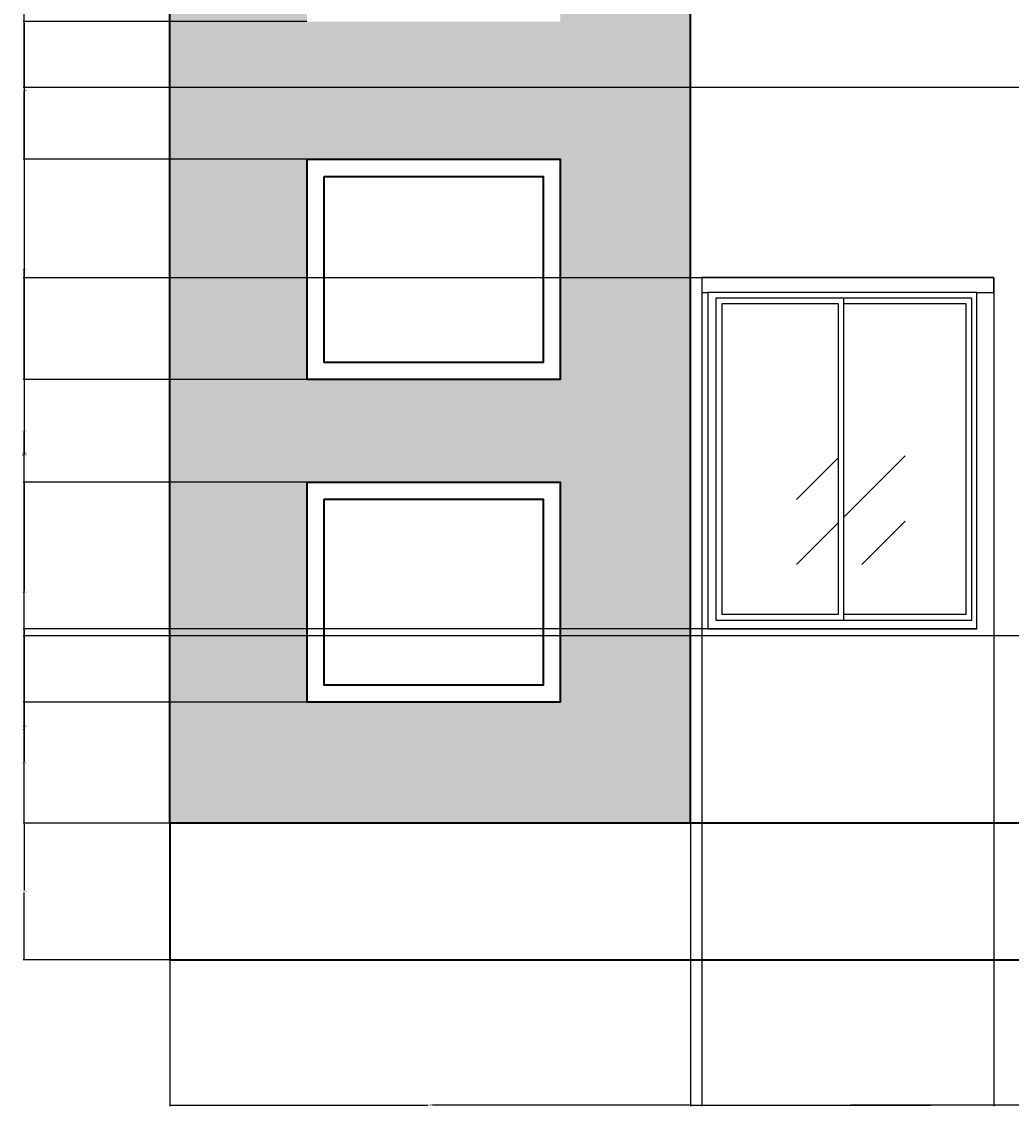
# Model space of a CAD drawing. Units: inches. Extents: x 93 to 565, y 123 to 656.
# Tile 1 of 18: x 93 to 267, y 134 to 324. Entities that reach past the tile are written whole.
import ezdxf

# ---------------------------------------------------------------- set-up
doc = ezdxf.new("R2010")
doc.units = ezdxf.units.IN
doc.header["$MEASUREMENT"] = 0
for name, color, linetype, lineweight in [('A-ANNO-DIMS', 2, 'Continuous', 18), ('A-ELEV', 7, 'Continuous', 35), ('A-GLAZ', 4, 'Continuous', 25), ('A-WALL-PATT', 8, 'Continuous', 13)]:
    doc.layers.add(name, color=color, linetype=linetype, lineweight=lineweight)
doc.styles.get("Standard").update_dxf_attribs({"font": 'arial.ttf'})
doc.dimstyles.get("Standard").update_dxf_attribs({"dimtxt": 0.18, "dimasz": 0.18, "dimexe": 0.18, "dimexo": 0.0625, "dimgap": 0.09, "dimtad": 0, "dimtih": 1, "dimtoh": 1, "dimdec": 4, "dimzin": 0, "dimdsep": 46, "dimtxsty": 'Standard', "dimcen": 0.09, "dimadec": 0, "dimazin": 0, "dimtfac": 1, "dimtdec": 4, "dimtofl": 0, "dimtmove": 0, "dimatfit": 3, "dimfxl": 1, "dimtolj": 1, "dimtzin": 0, "dimarcsym": 0})

# ---------------------------------------------------------------- blocks, each defined once
blk = doc.blocks.new('*U6')
for p, q in [((38.1, 38.1), (38.1, 1476.3)), ((38.1, 1476.3), (607.2, 1476.3)), ((607.2, 38.1), (607.2, 1476.3)), ((607.2, 1476.3), (1176.3, 1476.3)), ((1176.3, 1476.3), (1176.3, 38.1)), ((607.2, 38.1), (38.1, 38.1)), ((1176.3, 38.1), (607.2, 38.1))]:
    blk.add_line(p, q)
blk.add_lwpolyline([(0, 0), (1200, 0), (1200, 1500), (0, 1500)], close=True)
for points in [[(581.8, 1450.9), (581.8, 63.5), (63.5, 63.5), (63.5, 1450.9), (581.8, 1450.9)], [(607.2, 1450.9), (1150.9, 1450.9), (1150.9, 63.5), (607.2, 63.5)]]:
    blk.add_lwpolyline(points)
blk = doc.blocks.new('*D27')
at = {"layer": 'A-ANNO-DIMS', "color": 0, "lineweight": -2, "transparency": 16777216}
for p, q in [((210.54, 519.04), (210.54, 134)), ((119.08, 159.67), (119.08, 134)), ((119.26, 134.18), (164.42, 134.18)), ((210.36, 134.18), (165.21, 134.18))]:
    blk.add_line(p, q, dxfattribs=at)
at = {"layer": 'A-ANNO-DIMS', "color": 0, "transparency": 16777216}
for points in [[(119.26, 134.21), (119.26, 134.15), (119.08, 134.18)], [(210.36, 134.21), (210.36, 134.15), (210.54, 134.18)]]:
    blk.add_solid(points, dxfattribs=at)
at = {"layer": 'Defpoints', "color": 0, "transparency": 16777216}
for p in [(210.54, 519.1), (119.08, 159.73), (210.54, 134.18)]:
    blk.add_point(p, dxfattribs=at)
at = {"layer": 'A-ANNO-DIMS', "color": 0, "transparency": 16777216, "insert": (164.81, 134.18), "char_height": 0.18, "attachment_point": 5}
blk.add_mtext('\\A1;91.46', dxfattribs=at)
blk = doc.blocks.new('*D28')
at = {"layer": 'A-ANNO-DIMS', "color": 0, "lineweight": -2, "transparency": 16777216}
for p, q in [((210.54, 519.04), (210.54, 134)), ((295.69, 183.67), (295.69, 134)), ((210.72, 134.18), (252.72, 134.18)), ((295.51, 134.18), (253.51, 134.18))]:
    blk.add_line(p, q, dxfattribs=at)
at = {"layer": 'A-ANNO-DIMS', "color": 0, "transparency": 16777216}
for points in [[(210.72, 134.21), (210.72, 134.15), (210.54, 134.18)], [(295.51, 134.21), (295.51, 134.15), (295.69, 134.18)]]:
    blk.add_solid(points, dxfattribs=at)
at = {"layer": 'Defpoints', "color": 0, "transparency": 16777216}
for p in [(210.54, 519.1), (295.69, 183.73), (295.69, 134.18)]:
    blk.add_point(p, dxfattribs=at)
at = {"layer": 'A-ANNO-DIMS', "color": 0, "transparency": 16777216, "insert": (253.12, 134.18), "char_height": 0.18, "attachment_point": 5}
blk.add_mtext('\\A1;85.14', dxfattribs=at)
blk = doc.blocks.new('*D31')
at = {"layer": 'A-ANNO-DIMS', "color": 0, "lineweight": -2, "transparency": 16777216}
for p, q in [((417.87, 630.4), (564.81, 630.4)), ((564.63, 630.22), (564.63, 395.25)), ((564.63, 159.91), (564.63, 394.89)), ((119.14, 159.73), (564.81, 159.73))]:
    blk.add_line(p, q, dxfattribs=at)
at = {"layer": 'A-ANNO-DIMS', "color": 0, "transparency": 16777216}
for points in [[(564.6, 630.22), (564.66, 630.22), (564.63, 630.4)], [(564.6, 159.91), (564.66, 159.91), (564.63, 159.73)]]:
    blk.add_solid(points, dxfattribs=at)
at = {"layer": 'Defpoints', "color": 0, "transparency": 16777216}
for p in [(417.81, 630.4), (564.63, 630.4), (119.08, 159.73)]:
    blk.add_point(p, dxfattribs=at)
at = {"layer": 'A-ANNO-DIMS', "color": 0, "transparency": 16777216, "insert": (564.63, 395.07), "char_height": 0.18, "attachment_point": 5}
blk.add_mtext('\\A1;470.7', dxfattribs=at)
blk = doc.blocks.new('*D32')
at = {"layer": 'A-ANNO-DIMS', "color": 0, "lineweight": -2, "transparency": 16777216}
for p, q in [((119.02, 183.73), (93.35, 183.73)), ((93.53, 183.55), (93.53, 171.91)), ((93.53, 159.91), (93.53, 171.55)), ((119.02, 159.73), (93.35, 159.73))]:
    blk.add_line(p, q, dxfattribs=at)
at = {"layer": 'A-ANNO-DIMS', "color": 0, "transparency": 16777216}
for points in [[(93.5, 183.55), (93.56, 183.55), (93.53, 183.73)], [(93.5, 159.91), (93.56, 159.91), (93.53, 159.73)]]:
    blk.add_solid(points, dxfattribs=at)
at = {"layer": 'Defpoints', "color": 0, "transparency": 16777216}
for p in [(93.53, 183.73), (119.08, 183.73), (119.08, 159.73)]:
    blk.add_point(p, dxfattribs=at)
at = {"layer": 'A-ANNO-DIMS', "color": 0, "transparency": 16777216, "insert": (93.53, 171.73), "char_height": 0.18, "attachment_point": 5}
blk.add_mtext('\\A1;24', dxfattribs=at)
blk = doc.blocks.new('*D33')
at = {"layer": 'A-ANNO-DIMS', "color": 0, "lineweight": -2, "transparency": 16777216}
for p, q in [((286.62, 312.95), (93.35, 312.95)), ((93.53, 312.77), (93.53, 248.52)), ((93.53, 183.91), (93.53, 248.16)), ((119.02, 183.73), (93.35, 183.73))]:
    blk.add_line(p, q, dxfattribs=at)
at = {"layer": 'A-ANNO-DIMS', "color": 0, "transparency": 16777216}
for points in [[(93.5, 312.77), (93.56, 312.77), (93.53, 312.95)], [(93.5, 183.91), (93.56, 183.91), (93.53, 183.73)]]:
    blk.add_solid(points, dxfattribs=at)
at = {"layer": 'Defpoints', "color": 0, "transparency": 16777216}
for p in [(93.53, 312.95), (286.69, 312.95), (119.08, 183.73)]:
    blk.add_point(p, dxfattribs=at)
at = {"layer": 'A-ANNO-DIMS', "color": 0, "transparency": 16777216, "insert": (93.53, 248.34), "char_height": 0.18, "attachment_point": 5}
blk.add_mtext('\\A1;129.22', dxfattribs=at)
blk = doc.blocks.new('*D34')
at = {"layer": 'A-ANNO-DIMS', "color": 0, "lineweight": -2, "transparency": 16777216}
for p, q in [((286.62, 363.73), (93.35, 363.73)), ((93.53, 363.55), (93.53, 338.52)), ((93.53, 313.13), (93.53, 338.16)), ((286.62, 312.95), (93.35, 312.95))]:
    blk.add_line(p, q, dxfattribs=at)
at = {"layer": 'A-ANNO-DIMS', "color": 0, "transparency": 16777216}
for points in [[(93.5, 363.55), (93.56, 363.55), (93.53, 363.73)], [(93.5, 313.13), (93.56, 313.13), (93.53, 312.95)]]:
    blk.add_solid(points, dxfattribs=at)
at = {"layer": 'Defpoints', "color": 0, "transparency": 16777216}
for p in [(93.53, 363.73), (286.69, 363.73), (286.69, 312.95)]:
    blk.add_point(p, dxfattribs=at)
at = {"layer": 'A-ANNO-DIMS', "color": 0, "transparency": 16777216, "insert": (93.53, 338.34), "char_height": 0.18, "attachment_point": 5}
blk.add_mtext('\\A1;50.78', dxfattribs=at)
blk = doc.blocks.new('*D38')
at = {"layer": 'A-ANNO-DIMS', "color": 0, "lineweight": -2, "transparency": 16777216}
for p, q in [((143.15, 204.96), (93.35, 204.96)), ((93.53, 204.78), (93.53, 194.53)), ((93.53, 183.91), (93.53, 194.16)), ((210.48, 183.73), (93.35, 183.73))]:
    blk.add_line(p, q, dxfattribs=at)
at = {"layer": 'A-ANNO-DIMS', "color": 0, "transparency": 16777216}
for points in [[(93.5, 204.78), (93.56, 204.78), (93.53, 204.96)], [(93.5, 183.91), (93.56, 183.91), (93.53, 183.73)]]:
    blk.add_solid(points, dxfattribs=at)
at = {"layer": 'Defpoints', "color": 0, "transparency": 16777216}
for p in [(93.53, 204.96), (143.21, 204.96), (210.54, 183.73)]:
    blk.add_point(p, dxfattribs=at)
at = {"layer": 'A-ANNO-DIMS', "color": 0, "transparency": 16777216, "insert": (93.53, 194.35), "char_height": 0.18, "attachment_point": 5}
blk.add_mtext('\\A1;21.226', dxfattribs=at)
blk = doc.blocks.new('*D39')
at = {"layer": 'A-ANNO-DIMS', "color": 0, "lineweight": -2, "transparency": 16777216}
for p, q in [((143.15, 243.64), (93.35, 243.64)), ((93.53, 243.46), (93.53, 224.48)), ((93.53, 205.14), (93.53, 224.12)), ((143.15, 204.96), (93.35, 204.96))]:
    blk.add_line(p, q, dxfattribs=at)
at = {"layer": 'A-ANNO-DIMS', "color": 0, "transparency": 16777216}
for points in [[(93.5, 243.46), (93.56, 243.46), (93.53, 243.64)], [(93.5, 205.14), (93.56, 205.14), (93.53, 204.96)]]:
    blk.add_solid(points, dxfattribs=at)
at = {"layer": 'Defpoints', "color": 0, "transparency": 16777216}
for p in [(93.53, 243.64), (143.21, 243.64), (143.21, 204.96)]:
    blk.add_point(p, dxfattribs=at)
at = {"layer": 'A-ANNO-DIMS', "color": 0, "transparency": 16777216, "insert": (93.53, 224.3), "char_height": 0.18, "attachment_point": 5}
blk.add_mtext('\\A1;38.685', dxfattribs=at)
blk = doc.blocks.new('*D40')
at = {"layer": 'A-ANNO-DIMS', "color": 0, "lineweight": -2, "transparency": 16777216}
for p, q in [((143.15, 261.64), (93.35, 261.64)), ((93.53, 261.46), (93.53, 252.82)), ((93.53, 243.82), (93.53, 252.46)), ((143.15, 243.64), (93.35, 243.64))]:
    blk.add_line(p, q, dxfattribs=at)
at = {"layer": 'A-ANNO-DIMS', "color": 0, "transparency": 16777216}
for points in [[(93.5, 261.46), (93.56, 261.46), (93.53, 261.64)], [(93.5, 243.82), (93.56, 243.82), (93.53, 243.64)]]:
    blk.add_solid(points, dxfattribs=at)
at = {"layer": 'Defpoints', "color": 0, "transparency": 16777216}
for p in [(93.53, 261.64), (143.21, 261.64), (143.21, 243.64)]:
    blk.add_point(p, dxfattribs=at)
at = {"layer": 'A-ANNO-DIMS', "color": 0, "transparency": 16777216, "insert": (93.53, 252.64), "char_height": 0.18, "attachment_point": 5}
blk.add_mtext('\\A1;17.995', dxfattribs=at)
blk = doc.blocks.new('*D41')
at = {"layer": 'A-ANNO-DIMS', "color": 0, "lineweight": -2, "transparency": 16777216}
for p, q in [((143.15, 300.32), (93.35, 300.32)), ((93.53, 300.14), (93.53, 281.16)), ((93.53, 261.82), (93.53, 280.8)), ((143.15, 261.64), (93.35, 261.64))]:
    blk.add_line(p, q, dxfattribs=at)
at = {"layer": 'A-ANNO-DIMS', "color": 0, "transparency": 16777216}
for points in [[(93.5, 300.14), (93.56, 300.14), (93.53, 300.32)], [(93.5, 261.82), (93.56, 261.82), (93.53, 261.64)]]:
    blk.add_solid(points, dxfattribs=at)
at = {"layer": 'Defpoints', "color": 0, "transparency": 16777216}
for p in [(93.53, 300.32), (143.21, 300.32), (143.21, 261.64)]:
    blk.add_point(p, dxfattribs=at)
at = {"layer": 'A-ANNO-DIMS', "color": 0, "transparency": 16777216, "insert": (93.53, 280.98), "char_height": 0.18, "attachment_point": 5}
blk.add_mtext('\\A1;38.685', dxfattribs=at)
blk = doc.blocks.new('*D42')
at = {"layer": 'A-ANNO-DIMS', "color": 0, "lineweight": -2, "transparency": 16777216}
for p, q in [((143.15, 324.49), (93.35, 324.49)), ((93.53, 324.31), (93.53, 312.59)), ((93.53, 300.5), (93.53, 312.22)), ((143.15, 300.32), (93.35, 300.32))]:
    blk.add_line(p, q, dxfattribs=at)
at = {"layer": 'A-ANNO-DIMS', "color": 0, "transparency": 16777216}
for points in [[(93.5, 324.31), (93.56, 324.31), (93.53, 324.49)], [(93.5, 300.5), (93.56, 300.5), (93.53, 300.32)]]:
    blk.add_solid(points, dxfattribs=at)
at = {"layer": 'Defpoints', "color": 0, "transparency": 16777216}
for p in [(93.53, 324.49), (143.21, 324.49), (143.21, 300.32)]:
    blk.add_point(p, dxfattribs=at)
at = {"layer": 'A-ANNO-DIMS', "color": 0, "transparency": 16777216, "insert": (93.53, 312.4), "char_height": 0.18, "attachment_point": 5}
blk.add_mtext('\\A1;24.16', dxfattribs=at)
blk = doc.blocks.new('*D43')
at = {"layer": 'A-ANNO-DIMS', "color": 0, "lineweight": -2, "transparency": 16777216}
for p, q in [((143.15, 363.17), (93.35, 363.17)), ((93.53, 362.99), (93.53, 344.01)), ((93.53, 324.67), (93.53, 343.65)), ((143.15, 324.49), (93.35, 324.49))]:
    blk.add_line(p, q, dxfattribs=at)
at = {"layer": 'A-ANNO-DIMS', "color": 0, "transparency": 16777216}
for points in [[(93.5, 362.99), (93.56, 362.99), (93.53, 363.17)], [(93.5, 324.67), (93.56, 324.67), (93.53, 324.49)]]:
    blk.add_solid(points, dxfattribs=at)
at = {"layer": 'Defpoints', "color": 0, "transparency": 16777216}
for p in [(93.53, 363.17), (143.21, 363.17), (143.21, 324.49)]:
    blk.add_point(p, dxfattribs=at)
at = {"layer": 'A-ANNO-DIMS', "color": 0, "transparency": 16777216, "insert": (93.53, 343.83), "char_height": 0.18, "attachment_point": 5}
blk.add_mtext('\\A1;38.685', dxfattribs=at)
blk = doc.blocks.new('*D52')
at = {"layer": 'A-ANNO-DIMS', "color": 0, "lineweight": -2, "transparency": 16777216}
for p, q in [((212.49, 279.47), (212.49, 134)), ((263.81, 279.47), (263.81, 134)), ((212.67, 134.18), (237.76, 134.18)), ((263.63, 134.18), (238.54, 134.18))]:
    blk.add_line(p, q, dxfattribs=at)
at = {"layer": 'A-ANNO-DIMS', "color": 0, "transparency": 16777216}
for points in [[(212.67, 134.21), (212.67, 134.15), (212.49, 134.18)], [(263.63, 134.21), (263.63, 134.15), (263.81, 134.18)]]:
    blk.add_solid(points, dxfattribs=at)
at = {"layer": 'Defpoints', "color": 0, "transparency": 16777216}
for p in [(212.49, 279.53), (263.81, 279.53), (263.81, 134.18)]:
    blk.add_point(p, dxfattribs=at)
at = {"layer": 'A-ANNO-DIMS', "color": 0, "transparency": 16777216, "insert": (238.15, 134.18), "char_height": 0.18, "attachment_point": 5}
blk.add_mtext('\\A1;51.33', dxfattribs=at)
blk = doc.blocks.new('*D53')
at = {"layer": 'A-ANNO-DIMS', "color": 0, "lineweight": -2, "transparency": 16777216}
for p, q in [((263.75, 279.53), (93.35, 279.53)), ((93.53, 279.35), (93.53, 248.87)), ((93.53, 218.03), (93.53, 248.51)), ((260.74, 217.85), (93.35, 217.85))]:
    blk.add_line(p, q, dxfattribs=at)
at = {"layer": 'A-ANNO-DIMS', "color": 0, "transparency": 16777216}
for points in [[(93.5, 279.35), (93.56, 279.35), (93.53, 279.53)], [(93.5, 218.03), (93.56, 218.03), (93.53, 217.85)]]:
    blk.add_solid(points, dxfattribs=at)
at = {"layer": 'Defpoints', "color": 0, "transparency": 16777216}
for p in [(93.53, 279.53), (263.81, 279.53), (260.8, 217.85)]:
    blk.add_point(p, dxfattribs=at)
at = {"layer": 'A-ANNO-DIMS', "color": 0, "transparency": 16777216, "insert": (93.53, 248.69), "char_height": 0.18, "attachment_point": 5}
blk.add_mtext('\\A1;61.68', dxfattribs=at)
blk = doc.blocks.new('*D54')
at = {"layer": 'A-ANNO-DIMS', "color": 0, "lineweight": -2, "transparency": 16777216}
for p, q in [((213.49, 217.85), (93.35, 217.85)), ((93.53, 217.67), (93.53, 200.97)), ((93.53, 183.91), (93.53, 200.61)), ((210.48, 183.73), (93.35, 183.73))]:
    blk.add_line(p, q, dxfattribs=at)
at = {"layer": 'A-ANNO-DIMS', "color": 0, "transparency": 16777216}
for points in [[(93.5, 217.67), (93.56, 217.67), (93.53, 217.85)], [(93.5, 183.91), (93.56, 183.91), (93.53, 183.73)]]:
    blk.add_solid(points, dxfattribs=at)
at = {"layer": 'Defpoints', "color": 0, "transparency": 16777216}
for p in [(213.56, 217.85), (93.53, 183.73), (210.54, 183.73)]:
    blk.add_point(p, dxfattribs=at)
at = {"layer": 'A-ANNO-DIMS', "color": 0, "transparency": 16777216, "insert": (93.53, 200.79), "char_height": 0.18, "attachment_point": 5}
blk.add_mtext('\\A1;34.114', dxfattribs=at)
blk = doc.blocks.new('*D58')
at = {"layer": 'A-ANNO-DIMS', "color": 0, "lineweight": -2, "transparency": 16777216}
for p, q in [((309.68, 216.63), (93.35, 216.63)), ((93.53, 216.45), (93.53, 200.36)), ((93.53, 183.91), (93.53, 200)), ((295.62, 183.73), (93.35, 183.73))]:
    blk.add_line(p, q, dxfattribs=at)
at = {"layer": 'A-ANNO-DIMS', "color": 0, "transparency": 16777216}
for points in [[(93.5, 216.45), (93.56, 216.45), (93.53, 216.63)], [(93.5, 183.91), (93.56, 183.91), (93.53, 183.73)]]:
    blk.add_solid(points, dxfattribs=at)
at = {"layer": 'Defpoints', "color": 0, "transparency": 16777216}
for p in [(309.74, 216.63), (93.53, 183.73), (295.69, 183.73)]:
    blk.add_point(p, dxfattribs=at)
at = {"layer": 'A-ANNO-DIMS', "color": 0, "transparency": 16777216, "insert": (93.53, 200.18), "char_height": 0.18, "attachment_point": 5}
blk.add_mtext('\\A1;32.9', dxfattribs=at)
blk = doc.blocks.new('*D106')
at = {"layer": 'A-ANNO-DIMS', "color": 0, "lineweight": -2, "transparency": 16777216}
for p, q in [((210.54, 519.04), (210.54, 134)), ((119.08, 159.67), (119.08, 134)), ((119.26, 134.18), (164.35, 134.18)), ((210.36, 134.18), (165.28, 134.18))]:
    blk.add_line(p, q, dxfattribs=at)
at = {"layer": 'A-ANNO-DIMS', "color": 0, "transparency": 16777216}
for points in [[(119.26, 134.21), (119.26, 134.15), (119.08, 134.18)], [(210.36, 134.21), (210.36, 134.15), (210.54, 134.18)]]:
    blk.add_solid(points, dxfattribs=at)
at = {"layer": 'Defpoints', "color": 0, "transparency": 16777216}
for p in [(210.54, 519.1), (119.08, 159.73), (210.54, 134.18)]:
    blk.add_point(p, dxfattribs=at)
at = {"layer": 'A-ANNO-DIMS', "color": 0, "transparency": 16777216, "insert": (164.81, 134.18), "char_height": 0.18, "attachment_point": 5}
blk.add_mtext('\\A1;91.465', dxfattribs=at)
blk = doc.blocks.new('*D107')
at = {"layer": 'A-ANNO-DIMS', "color": 0, "lineweight": -2, "transparency": 16777216}
for p, q in [((210.54, 519.04), (210.54, 134)), ((295.69, 183.67), (295.69, 134)), ((210.72, 134.18), (252.65, 134.18)), ((295.51, 134.18), (253.58, 134.18))]:
    blk.add_line(p, q, dxfattribs=at)
at = {"layer": 'A-ANNO-DIMS', "color": 0, "transparency": 16777216}
for points in [[(210.72, 134.21), (210.72, 134.15), (210.54, 134.18)], [(295.51, 134.21), (295.51, 134.15), (295.69, 134.18)]]:
    blk.add_solid(points, dxfattribs=at)
at = {"layer": 'Defpoints', "color": 0, "transparency": 16777216}
for p in [(210.54, 519.1), (295.69, 183.73), (295.69, 134.18)]:
    blk.add_point(p, dxfattribs=at)
at = {"layer": 'A-ANNO-DIMS', "color": 0, "transparency": 16777216, "insert": (253.12, 134.18), "char_height": 0.18, "attachment_point": 5}
blk.add_mtext('\\A1;85.143', dxfattribs=at)
blk = doc.blocks.new('*D110')
at = {"layer": 'A-ANNO-DIMS', "color": 0, "lineweight": -2, "transparency": 16777216}
for p, q in [((417.87, 630.4), (564.81, 630.4)), ((564.63, 630.22), (564.63, 395.25)), ((564.63, 159.91), (564.63, 394.89)), ((119.14, 159.73), (564.81, 159.73))]:
    blk.add_line(p, q, dxfattribs=at)
at = {"layer": 'A-ANNO-DIMS', "color": 0, "transparency": 16777216}
for points in [[(564.6, 630.22), (564.66, 630.22), (564.63, 630.4)], [(564.6, 159.91), (564.66, 159.91), (564.63, 159.73)]]:
    blk.add_solid(points, dxfattribs=at)
at = {"layer": 'Defpoints', "color": 0, "transparency": 16777216}
for p in [(417.81, 630.4), (564.63, 630.4), (119.08, 159.73)]:
    blk.add_point(p, dxfattribs=at)
at = {"layer": 'A-ANNO-DIMS', "color": 0, "transparency": 16777216, "insert": (564.63, 395.07), "char_height": 0.18, "attachment_point": 5}
blk.add_mtext('\\A1;470.673', dxfattribs=at)
blk = doc.blocks.new('*D111')
at = {"layer": 'A-ANNO-DIMS', "color": 0, "lineweight": -2, "transparency": 16777216}
for p, q in [((119.02, 183.73), (93.35, 183.73)), ((93.53, 183.55), (93.53, 171.91)), ((93.53, 159.91), (93.53, 171.55)), ((119.02, 159.73), (93.35, 159.73))]:
    blk.add_line(p, q, dxfattribs=at)
at = {"layer": 'A-ANNO-DIMS', "color": 0, "transparency": 16777216}
for points in [[(93.5, 183.55), (93.56, 183.55), (93.53, 183.73)], [(93.5, 159.91), (93.56, 159.91), (93.53, 159.73)]]:
    blk.add_solid(points, dxfattribs=at)
at = {"layer": 'Defpoints', "color": 0, "transparency": 16777216}
for p in [(93.53, 183.73), (119.08, 183.73), (119.08, 159.73)]:
    blk.add_point(p, dxfattribs=at)
at = {"layer": 'A-ANNO-DIMS', "color": 0, "transparency": 16777216, "insert": (93.53, 171.73), "char_height": 0.18, "attachment_point": 5}
blk.add_mtext('\\A1;24.000', dxfattribs=at)
blk = doc.blocks.new('*D112')
at = {"layer": 'A-ANNO-DIMS', "color": 0, "lineweight": -2, "transparency": 16777216}
for p, q in [((286.62, 312.95), (93.35, 312.95)), ((93.53, 312.77), (93.53, 248.52)), ((93.53, 183.91), (93.53, 248.16)), ((119.02, 183.73), (93.35, 183.73))]:
    blk.add_line(p, q, dxfattribs=at)
at = {"layer": 'A-ANNO-DIMS', "color": 0, "transparency": 16777216}
for points in [[(93.5, 312.77), (93.56, 312.77), (93.53, 312.95)], [(93.5, 183.91), (93.56, 183.91), (93.53, 183.73)]]:
    blk.add_solid(points, dxfattribs=at)
at = {"layer": 'Defpoints', "color": 0, "transparency": 16777216}
for p in [(93.53, 312.95), (286.69, 312.95), (119.08, 183.73)]:
    blk.add_point(p, dxfattribs=at)
at = {"layer": 'A-ANNO-DIMS', "color": 0, "transparency": 16777216, "insert": (93.53, 248.34), "char_height": 0.18, "attachment_point": 5}
blk.add_mtext('\\A1;129.217', dxfattribs=at)
blk = doc.blocks.new('*D113')
at = {"layer": 'A-ANNO-DIMS', "color": 0, "lineweight": -2, "transparency": 16777216}
for p, q in [((286.62, 363.73), (93.35, 363.73)), ((93.53, 363.55), (93.53, 338.52)), ((93.53, 313.13), (93.53, 338.16)), ((286.62, 312.95), (93.35, 312.95))]:
    blk.add_line(p, q, dxfattribs=at)
at = {"layer": 'A-ANNO-DIMS', "color": 0, "transparency": 16777216}
for points in [[(93.5, 363.55), (93.56, 363.55), (93.53, 363.73)], [(93.5, 313.13), (93.56, 313.13), (93.53, 312.95)]]:
    blk.add_solid(points, dxfattribs=at)
at = {"layer": 'Defpoints', "color": 0, "transparency": 16777216}
for p in [(93.53, 363.73), (286.69, 363.73), (286.69, 312.95)]:
    blk.add_point(p, dxfattribs=at)
at = {"layer": 'A-ANNO-DIMS', "color": 0, "transparency": 16777216, "insert": (93.53, 338.34), "char_height": 0.18, "attachment_point": 5}
blk.add_mtext('\\A1;50.783', dxfattribs=at)
blk = doc.blocks.new('*D117')
at = {"layer": 'A-ANNO-DIMS', "color": 0, "lineweight": -2, "transparency": 16777216}
for p, q in [((143.15, 204.96), (93.35, 204.96)), ((93.53, 204.78), (93.53, 194.53)), ((93.53, 183.91), (93.53, 194.16)), ((210.48, 183.73), (93.35, 183.73))]:
    blk.add_line(p, q, dxfattribs=at)
at = {"layer": 'A-ANNO-DIMS', "color": 0, "transparency": 16777216}
for points in [[(93.5, 204.78), (93.56, 204.78), (93.53, 204.96)], [(93.5, 183.91), (93.56, 183.91), (93.53, 183.73)]]:
    blk.add_solid(points, dxfattribs=at)
at = {"layer": 'Defpoints', "color": 0, "transparency": 16777216}
for p in [(93.53, 204.96), (143.21, 204.96), (210.54, 183.73)]:
    blk.add_point(p, dxfattribs=at)
at = {"layer": 'A-ANNO-DIMS', "color": 0, "transparency": 16777216, "insert": (93.53, 194.35), "char_height": 0.18, "attachment_point": 5}
blk.add_mtext('\\A1;21.226', dxfattribs=at)
blk = doc.blocks.new('*D118')
at = {"layer": 'A-ANNO-DIMS', "color": 0, "lineweight": -2, "transparency": 16777216}
for p, q in [((143.15, 243.64), (93.35, 243.64)), ((93.53, 243.46), (93.53, 224.48)), ((93.53, 205.14), (93.53, 224.12)), ((143.15, 204.96), (93.35, 204.96))]:
    blk.add_line(p, q, dxfattribs=at)
at = {"layer": 'A-ANNO-DIMS', "color": 0, "transparency": 16777216}
for points in [[(93.5, 243.46), (93.56, 243.46), (93.53, 243.64)], [(93.5, 205.14), (93.56, 205.14), (93.53, 204.96)]]:
    blk.add_solid(points, dxfattribs=at)
at = {"layer": 'Defpoints', "color": 0, "transparency": 16777216}
for p in [(93.53, 243.64), (143.21, 243.64), (143.21, 204.96)]:
    blk.add_point(p, dxfattribs=at)
at = {"layer": 'A-ANNO-DIMS', "color": 0, "transparency": 16777216, "insert": (93.53, 224.3), "char_height": 0.18, "attachment_point": 5}
blk.add_mtext('\\A1;38.685', dxfattribs=at)
blk = doc.blocks.new('*D119')
at = {"layer": 'A-ANNO-DIMS', "color": 0, "lineweight": -2, "transparency": 16777216}
for p, q in [((143.15, 261.64), (93.35, 261.64)), ((93.53, 261.46), (93.53, 252.82)), ((93.53, 243.82), (93.53, 252.46)), ((143.15, 243.64), (93.35, 243.64))]:
    blk.add_line(p, q, dxfattribs=at)
at = {"layer": 'A-ANNO-DIMS', "color": 0, "transparency": 16777216}
for points in [[(93.5, 261.46), (93.56, 261.46), (93.53, 261.64)], [(93.5, 243.82), (93.56, 243.82), (93.53, 243.64)]]:
    blk.add_solid(points, dxfattribs=at)
at = {"layer": 'Defpoints', "color": 0, "transparency": 16777216}
for p in [(93.53, 261.64), (143.21, 261.64), (143.21, 243.64)]:
    blk.add_point(p, dxfattribs=at)
at = {"layer": 'A-ANNO-DIMS', "color": 0, "transparency": 16777216, "insert": (93.53, 252.64), "char_height": 0.18, "attachment_point": 5}
blk.add_mtext('\\A1;17.995', dxfattribs=at)
blk = doc.blocks.new('*D120')
at = {"layer": 'A-ANNO-DIMS', "color": 0, "lineweight": -2, "transparency": 16777216}
for p, q in [((143.15, 300.32), (93.35, 300.32)), ((93.53, 300.14), (93.53, 281.16)), ((93.53, 261.82), (93.53, 280.8)), ((143.15, 261.64), (93.35, 261.64))]:
    blk.add_line(p, q, dxfattribs=at)
at = {"layer": 'A-ANNO-DIMS', "color": 0, "transparency": 16777216}
for points in [[(93.5, 300.14), (93.56, 300.14), (93.53, 300.32)], [(93.5, 261.82), (93.56, 261.82), (93.53, 261.64)]]:
    blk.add_solid(points, dxfattribs=at)
at = {"layer": 'Defpoints', "color": 0, "transparency": 16777216}
for p in [(93.53, 300.32), (143.21, 300.32), (143.21, 261.64)]:
    blk.add_point(p, dxfattribs=at)
at = {"layer": 'A-ANNO-DIMS', "color": 0, "transparency": 16777216, "insert": (93.53, 280.98), "char_height": 0.18, "attachment_point": 5}
blk.add_mtext('\\A1;38.685', dxfattribs=at)
blk = doc.blocks.new('*D121')
at = {"layer": 'A-ANNO-DIMS', "color": 0, "lineweight": -2, "transparency": 16777216}
for p, q in [((143.15, 324.49), (93.35, 324.49)), ((93.53, 324.31), (93.53, 312.59)), ((93.53, 300.5), (93.53, 312.22)), ((143.15, 300.32), (93.35, 300.32))]:
    blk.add_line(p, q, dxfattribs=at)
at = {"layer": 'A-ANNO-DIMS', "color": 0, "transparency": 16777216}
for points in [[(93.5, 324.31), (93.56, 324.31), (93.53, 324.49)], [(93.5, 300.5), (93.56, 300.5), (93.53, 300.32)]]:
    blk.add_solid(points, dxfattribs=at)
at = {"layer": 'Defpoints', "color": 0, "transparency": 16777216}
for p in [(93.53, 324.49), (143.21, 324.49), (143.21, 300.32)]:
    blk.add_point(p, dxfattribs=at)
at = {"layer": 'A-ANNO-DIMS', "color": 0, "transparency": 16777216, "insert": (93.53, 312.4), "char_height": 0.18, "attachment_point": 5}
blk.add_mtext('\\A1;24.160', dxfattribs=at)
blk = doc.blocks.new('*D122')
at = {"layer": 'A-ANNO-DIMS', "color": 0, "lineweight": -2, "transparency": 16777216}
for p, q in [((143.15, 363.17), (93.35, 363.17)), ((93.53, 362.99), (93.53, 344.01)), ((93.53, 324.67), (93.53, 343.65)), ((143.15, 324.49), (93.35, 324.49))]:
    blk.add_line(p, q, dxfattribs=at)
at = {"layer": 'A-ANNO-DIMS', "color": 0, "transparency": 16777216}
for points in [[(93.5, 362.99), (93.56, 362.99), (93.53, 363.17)], [(93.5, 324.67), (93.56, 324.67), (93.53, 324.49)]]:
    blk.add_solid(points, dxfattribs=at)
at = {"layer": 'Defpoints', "color": 0, "transparency": 16777216}
for p in [(93.53, 363.17), (143.21, 363.17), (143.21, 324.49)]:
    blk.add_point(p, dxfattribs=at)
at = {"layer": 'A-ANNO-DIMS', "color": 0, "transparency": 16777216, "insert": (93.53, 343.83), "char_height": 0.18, "attachment_point": 5}
blk.add_mtext('\\A1;38.685', dxfattribs=at)
blk = doc.blocks.new('*D131')
at = {"layer": 'A-ANNO-DIMS', "color": 0, "lineweight": -2, "transparency": 16777216}
for p, q in [((212.49, 279.47), (212.49, 134)), ((263.81, 279.47), (263.81, 134)), ((212.67, 134.18), (237.69, 134.18)), ((263.63, 134.18), (238.61, 134.18))]:
    blk.add_line(p, q, dxfattribs=at)
at = {"layer": 'A-ANNO-DIMS', "color": 0, "transparency": 16777216}
for points in [[(212.67, 134.21), (212.67, 134.15), (212.49, 134.18)], [(263.63, 134.21), (263.63, 134.15), (263.81, 134.18)]]:
    blk.add_solid(points, dxfattribs=at)
at = {"layer": 'Defpoints', "color": 0, "transparency": 16777216}
for p in [(212.49, 279.53), (263.81, 279.53), (263.81, 134.18)]:
    blk.add_point(p, dxfattribs=at)
at = {"layer": 'A-ANNO-DIMS', "color": 0, "transparency": 16777216, "insert": (238.15, 134.18), "char_height": 0.18, "attachment_point": 5}
blk.add_mtext('\\A1;51.327', dxfattribs=at)
blk = doc.blocks.new('*D132')
at = {"layer": 'A-ANNO-DIMS', "color": 0, "lineweight": -2, "transparency": 16777216}
for p, q in [((263.75, 279.53), (93.35, 279.53)), ((93.53, 279.35), (93.53, 248.87)), ((93.53, 218.03), (93.53, 248.51)), ((260.74, 217.85), (93.35, 217.85))]:
    blk.add_line(p, q, dxfattribs=at)
at = {"layer": 'A-ANNO-DIMS', "color": 0, "transparency": 16777216}
for points in [[(93.5, 279.35), (93.56, 279.35), (93.53, 279.53)], [(93.5, 218.03), (93.56, 218.03), (93.53, 217.85)]]:
    blk.add_solid(points, dxfattribs=at)
at = {"layer": 'Defpoints', "color": 0, "transparency": 16777216}
for p in [(93.53, 279.53), (263.81, 279.53), (260.8, 217.85)]:
    blk.add_point(p, dxfattribs=at)
at = {"layer": 'A-ANNO-DIMS', "color": 0, "transparency": 16777216, "insert": (93.53, 248.69), "char_height": 0.18, "attachment_point": 5}
blk.add_mtext('\\A1;61.684', dxfattribs=at)
blk = doc.blocks.new('*D133')
at = {"layer": 'A-ANNO-DIMS', "color": 0, "lineweight": -2, "transparency": 16777216}
for p, q in [((213.49, 217.85), (93.35, 217.85)), ((93.53, 217.67), (93.53, 200.97)), ((93.53, 183.91), (93.53, 200.61)), ((210.48, 183.73), (93.35, 183.73))]:
    blk.add_line(p, q, dxfattribs=at)
at = {"layer": 'A-ANNO-DIMS', "color": 0, "transparency": 16777216}
for points in [[(93.5, 217.67), (93.56, 217.67), (93.53, 217.85)], [(93.5, 183.91), (93.56, 183.91), (93.53, 183.73)]]:
    blk.add_solid(points, dxfattribs=at)
at = {"layer": 'Defpoints', "color": 0, "transparency": 16777216}
for p in [(213.56, 217.85), (93.53, 183.73), (210.54, 183.73)]:
    blk.add_point(p, dxfattribs=at)
at = {"layer": 'A-ANNO-DIMS', "color": 0, "transparency": 16777216, "insert": (93.53, 200.79), "char_height": 0.18, "attachment_point": 5}
blk.add_mtext('\\A1;34.114', dxfattribs=at)
blk = doc.blocks.new('*D137')
at = {"layer": 'A-ANNO-DIMS', "color": 0, "lineweight": -2, "transparency": 16777216}
for p, q in [((309.68, 216.63), (93.35, 216.63)), ((93.53, 216.45), (93.53, 200.36)), ((93.53, 183.91), (93.53, 200)), ((295.62, 183.73), (93.35, 183.73))]:
    blk.add_line(p, q, dxfattribs=at)
at = {"layer": 'A-ANNO-DIMS', "color": 0, "transparency": 16777216}
for points in [[(93.5, 216.45), (93.56, 216.45), (93.53, 216.63)], [(93.5, 183.91), (93.56, 183.91), (93.53, 183.73)]]:
    blk.add_solid(points, dxfattribs=at)
at = {"layer": 'Defpoints', "color": 0, "transparency": 16777216}
for p in [(309.74, 216.63), (93.53, 183.73), (295.69, 183.73)]:
    blk.add_point(p, dxfattribs=at)
at = {"layer": 'A-ANNO-DIMS', "color": 0, "transparency": 16777216, "insert": (93.53, 200.18), "char_height": 0.18, "attachment_point": 5}
blk.add_mtext('\\A1;32.897', dxfattribs=at)

msp = doc.modelspace()

# ---------------------------------------------------------------- hatches: boundary and pattern name
at = {"layer": 'A-GLAZ'}
h = msp.add_hatch(dxfattribs=at)
h.set_pattern_fill('GOST_GLASS', color=256, scale=5.4)
h.set_pattern_definition([(45, (0, 0), (45.8205, 0), [27, -37.8]), (45, (11.455, 0), (45.8205, 0), [10.8, -54]), (45, (0, 11.455), (45.8205, 0), [10.8, -54])])
h.paths.add_polyline_path([(236.4617, 274.9686), (216.0562, 274.9686), (216.0562, 220.3466), (236.4617, 220.3466)])
h.paths.add_polyline_path([(258.8673, 274.9686), (237.4617, 274.9686), (237.4617, 220.3466), (258.8673, 220.3466)])
h.paths.add_polyline_path([(332.6288, 267.5414), (312.4161, 267.5414), (312.4161, 222.941), (332.6288, 222.941)])
h.paths.add_polyline_path([(366.6285, 270.8489), (341.2098, 270.8489), (341.2098, 220.4891), (366.6285, 220.4891)])
h.paths.add_polyline_path([(343.8825, 222.941), (364.0951, 222.941), (364.0951, 267.5414), (343.8825, 267.5414)], flags=16)
h.paths.add_polyline_path([(392.4256, 267.5414), (372.2129, 267.5414), (372.2129, 222.941), (392.4256, 222.941)])
h.paths.add_polyline_path([(421.7937, 267.5414), (401.581, 267.5414), (401.581, 222.941), (421.7937, 222.941)])
at = {"layer": 'A-WALL-PATT'}
h = msp.add_hatch(dxfattribs=at)
h.set_pattern_fill('STARS', color=256, scale=21)
h.paths.add_polyline_path([(210.5443, 507.7323), (210.5443, 519.0999), (119.0794, 519.0999), (119.0794, 507.7323), (119.0794, 183.7323), (210.5443, 183.7323)])
h.paths.add_polyline_path([(187.648, 430.1508), (187.648, 391.4653), (143.2118, 391.4653), (143.2118, 430.1508)], flags=16)
h.paths.add_polyline_path([(187.648, 455.6579), (143.2118, 455.6579), (143.2118, 494.3434), (187.648, 494.3434)], flags=16)
h.paths.add_polyline_path([(184.648, 427.1508), (184.648, 394.4653), (146.2118, 394.4653), (146.2118, 427.1508)], flags=0)
h.paths.add_polyline_path([(184.648, 458.6579), (146.2118, 458.6579), (146.2118, 491.3434), (184.648, 491.3434)], flags=0)
h.paths.add_polyline_path([(187.648, 363.1705), (187.648, 324.485), (143.2118, 324.485), (143.2118, 363.1705)], flags=16)
h.paths.add_polyline_path([(184.648, 360.1705), (184.648, 327.485), (146.2118, 327.485), (146.2118, 360.1705)], flags=0)
h.paths.add_polyline_path([(187.648, 300.3249), (187.648, 261.6394), (143.2118, 261.6394), (143.2118, 300.3249)], flags=16)
h.paths.add_polyline_path([(184.648, 297.3249), (184.648, 264.6394), (146.2118, 264.6394), (146.2118, 297.3249)], flags=0)
h.paths.add_polyline_path([(187.648, 243.6441), (187.648, 204.9587), (143.2118, 204.9587), (143.2118, 243.6441)], flags=16)
h.paths.add_polyline_path([(184.648, 240.6441), (184.648, 207.9587), (146.2118, 207.9587), (146.2118, 240.6441)], flags=0)

# ---------------------------------------------------------------- linework, layer by layer
at = {"layer": 'A-ELEV'}
for p, q in [((119.0794, 183.7323), (119.0794, 507.7323)), ((210.5443, 183.7323), (210.5443, 507.7323)), ((539.0794, 183.7323), (119.0794, 183.7323)), ((119.0794, 183.7323), (119.0794, 159.7323)), ((119.0794, 159.7323), (539.0794, 159.7323))]:
    msp.add_line(p, q, dxfattribs=at)
for points in [[(143.2118, 300.3249), (187.648, 300.3249), (187.648, 261.6394), (143.2118, 261.6394)], [(146.2118, 297.3249), (184.648, 297.3249), (184.648, 264.6394), (146.2118, 264.6394)], [(143.2118, 243.6441), (187.648, 243.6441), (187.648, 204.9587), (143.2118, 204.9587)], [(146.2118, 240.6441), (184.648, 240.6441), (184.648, 207.9587), (146.2118, 207.9587)]]:
    msp.add_lwpolyline(points, close=True, dxfattribs=at)
at = {"layer": 'A-GLAZ'}
for p, q in [((263.8123, 279.5308), (212.4856, 279.5308)), ((212.4856, 279.5308), (212.4856, 276.9017)), ((263.8123, 276.9017), (263.8123, 279.5308)), ((212.4856, 276.9017), (213.5562, 276.9017)), ((260.8003, 276.9017), (263.8123, 276.9017))]:
    msp.add_line(p, q, dxfattribs=at)

# ---------------------------------------------------------------- block references
at = {"layer": 'A-GLAZ', "xscale": 0.0393700787401575, "yscale": 0.0393700787401575, "zscale": 0.0393700787401575}
msp.add_blockref('*U6', (213.5562, 217.8466), dxfattribs=at)

# ---------------------------------------------------------------- dimensions: what is measured, and where the dimension line sits
at = {"layer": 'A-ANNO-DIMS'}
for base, p1, p2, override, picture, middle in [((564.6294, 630.4048), (119.0794, 159.7323), (417.8097, 630.4048), {"dimdec": 1, "dimlfac": 1, "dimrnd": 0, "dimzin": 0, "dimdsep": 46, "dimlunit": 2}, '*D31', (564.6294, 395.0685)), ((564.62936, 630.40478), (119.07936, 159.73225), (417.80971, 630.40477), {"dimdec": 3, "dimlfac": 1, "dimrnd": 0, "dimzin": 0, "dimdsep": 46, "dimlunit": 2}, '*D110', (564.62936, 395.06851)), ((93.5294, 363.7323), (286.6874, 312.9491), (286.6874, 363.7323), {"dimdec": 3, "dimlfac": 1, "dimrnd": 0, "dimzin": 0, "dimdsep": 46, "dimlunit": 2}, '*D113', (93.5294, 338.3407)), ((93.52936, 363.17052), (143.21177, 324.48505), (143.21177, 363.17052), {"dimdec": 3, "dimlfac": 1, "dimrnd": 0, "dimzin": 0, "dimdsep": 46, "dimlunit": 2}, '*D43', (93.52936, 343.82778)), ((93.52936, 363.17052), (143.21177, 324.48505), (143.21177, 363.17052), {"dimdec": 3, "dimlfac": 1, "dimrnd": 0, "dimzin": 0, "dimdsep": 46, "dimlunit": 2}, '*D122', (93.52936, 343.82778)), ((93.5294, 363.7323), (286.6874, 312.9491), (286.6874, 363.7323), {"dimdec": 2, "dimlfac": 1, "dimrnd": 0, "dimzin": 0, "dimdsep": 46, "dimlunit": 2}, '*D34', (93.5294, 338.3407)), ((93.5294, 324.485), (143.2118, 300.3249), (143.2118, 324.485), {"dimdec": 3, "dimlfac": 1, "dimrnd": 0, "dimzin": 0, "dimdsep": 46, "dimlunit": 2}, '*D121', (93.5294, 312.405)), ((93.5294, 324.485), (143.2118, 300.3249), (143.2118, 324.485), {"dimdec": 2, "dimlfac": 1, "dimrnd": 0, "dimzin": 0, "dimdsep": 46, "dimlunit": 2}, '*D42', (93.5294, 312.405)), ((93.5294, 312.9491), (119.0794, 183.7323), (286.6874, 312.9491), {"dimdec": 3, "dimlfac": 1, "dimrnd": 0, "dimzin": 0, "dimdsep": 46, "dimlunit": 2}, '*D112', (93.5294, 248.3407)), ((93.5294, 312.9491), (119.0794, 183.7323), (286.6874, 312.9491), {"dimdec": 2, "dimlfac": 1, "dimrnd": 0, "dimzin": 0, "dimdsep": 46, "dimlunit": 2}, '*D33', (93.5294, 248.3407)), ((93.52936, 300.32486), (143.21177, 261.63939), (143.21177, 300.32486), {"dimdec": 3, "dimlfac": 1, "dimrnd": 0, "dimzin": 0, "dimdsep": 46, "dimlunit": 2}, '*D41', (93.52936, 280.98212)), ((93.52936, 300.32486), (143.21177, 261.63939), (143.21177, 300.32486), {"dimdec": 3, "dimlfac": 1, "dimrnd": 0, "dimzin": 0, "dimdsep": 46, "dimlunit": 2}, '*D120', (93.52936, 280.98212)), ((93.5294, 279.5308), (260.8003, 217.8466), (263.8123, 279.5308), {"dimdec": 3, "dimlfac": 1, "dimrnd": 0, "dimzin": 0, "dimdsep": 46, "dimlunit": 2}, '*D132', (93.5294, 248.6887)), ((93.5294, 279.5308), (260.8003, 217.8466), (263.8123, 279.5308), {"dimdec": 2, "dimlfac": 1, "dimrnd": 0, "dimzin": 0, "dimdsep": 46, "dimlunit": 2}, '*D53', (93.5294, 248.6887)), ((93.5294, 261.6394), (143.2118, 243.6441), (143.2118, 261.6394), {"dimdec": 3, "dimlfac": 1, "dimrnd": 0, "dimzin": 0, "dimdsep": 46, "dimlunit": 2}, '*D40', (93.5294, 252.6418)), ((93.5294, 261.6394), (143.2118, 243.6441), (143.2118, 261.6394), {"dimdec": 3, "dimlfac": 1, "dimrnd": 0, "dimzin": 0, "dimdsep": 46, "dimlunit": 2}, '*D119', (93.5294, 252.6418)), ((93.5294, 243.6441), (143.2118, 204.9587), (143.2118, 243.6441), {"dimdec": 3, "dimlfac": 1, "dimrnd": 0, "dimzin": 0, "dimdsep": 46, "dimlunit": 2}, '*D39', (93.5294, 224.3014)), ((93.5294, 243.6441), (143.2118, 204.9587), (143.2118, 243.6441), {"dimdec": 3, "dimlfac": 1, "dimrnd": 0, "dimzin": 0, "dimdsep": 46, "dimlunit": 2}, '*D118', (93.5294, 224.3014)), ((93.5294, 183.7323), (213.5562, 217.8466), (210.5443, 183.7323), {"dimdec": 3, "dimlfac": 1, "dimrnd": 0, "dimzin": 0, "dimdsep": 46, "dimlunit": 2}, '*D54', (93.5294, 200.7894)), ((93.5294, 183.7323), (213.5562, 217.8466), (210.5443, 183.7323), {"dimdec": 3, "dimlfac": 1, "dimrnd": 0, "dimzin": 0, "dimdsep": 46, "dimlunit": 2}, '*D133', (93.5294, 200.7894)), ((93.5294, 183.7323), (309.7435, 216.6296), (295.6874, 183.7323), {"dimdec": 3, "dimlfac": 1, "dimrnd": 0, "dimzin": 0, "dimdsep": 46, "dimlunit": 2}, '*D137', (93.5294, 200.1809)), ((93.5294, 183.7323), (309.7435, 216.6296), (295.6874, 183.7323), {"dimdec": 1, "dimlfac": 1, "dimrnd": 0, "dimzin": 0, "dimdsep": 46, "dimlunit": 2}, '*D58', (93.5294, 200.1809)), ((93.5294, 204.9587), (210.5443, 183.7323), (143.2118, 204.9587), {"dimdec": 3, "dimlfac": 1, "dimrnd": 0, "dimzin": 0, "dimdsep": 46, "dimlunit": 2}, '*D38', (93.5294, 194.3455)), ((93.5294, 204.9587), (210.5443, 183.7323), (143.2118, 204.9587), {"dimdec": 3, "dimlfac": 1, "dimrnd": 0, "dimzin": 0, "dimdsep": 46, "dimlunit": 2}, '*D117', (93.5294, 194.3455)), ((93.5294, 183.7323), (119.0794, 159.7323), (119.0794, 183.7323), {"dimdec": 3, "dimlfac": 1, "dimrnd": 0, "dimzin": 0, "dimdsep": 46, "dimlunit": 2}, '*D111', (93.5294, 171.7323)), ((93.5294, 183.7323), (119.0794, 159.7323), (119.0794, 183.7323), {"dimdec": 0, "dimlfac": 1, "dimrnd": 0, "dimzin": 0, "dimdsep": 46, "dimlunit": 2}, '*D32', (93.5294, 171.7323))]:
    dim = msp.add_linear_dim(base=base, p1=p1, p2=p2, angle=90, dimstyle='Standard', override=override, dxfattribs=at)
    dim.commit()
    dim.dimension.update_dxf_attribs({"geometry": picture, "text_midpoint": middle})
for base, p1, p2, override, picture, middle in [((210.5443, 134.1823), (119.0794, 159.7323), (210.5443, 519.0999), {"dimdec": 2, "dimlfac": 1, "dimrnd": 0, "dimzin": 0, "dimdsep": 46, "dimlunit": 2}, '*D27', (164.8118, 134.1823)), ((210.5443, 134.1823), (119.0794, 159.7323), (210.5443, 519.0999), {"dimdec": 3, "dimlfac": 1, "dimrnd": 0, "dimzin": 0, "dimdsep": 46, "dimlunit": 2}, '*D106', (164.8118, 134.1823)), ((295.6874, 134.1823), (210.5443, 519.0999), (295.6874, 183.7323), {"dimdec": 2, "dimlfac": 1, "dimrnd": 0, "dimzin": 0, "dimdsep": 46, "dimlunit": 2}, '*D28', (253.1158, 134.1823)), ((295.6874, 134.1823), (210.5443, 519.0999), (295.6874, 183.7323), {"dimdec": 3, "dimlfac": 1, "dimrnd": 0, "dimzin": 0, "dimdsep": 46, "dimlunit": 2}, '*D107', (253.1158, 134.1823)), ((263.8123, 134.1823), (212.4856, 279.5308), (263.8123, 279.5308), {"dimdec": 2, "dimlfac": 1, "dimrnd": 0, "dimzin": 0, "dimdsep": 46, "dimlunit": 2}, '*D52', (238.1489, 134.1823)), ((263.8123, 134.1823), (212.4856, 279.5308), (263.8123, 279.5308), {"dimdec": 3, "dimlfac": 1, "dimrnd": 0, "dimzin": 0, "dimdsep": 46, "dimlunit": 2}, '*D131', (238.1489, 134.1823))]:
    dim = msp.add_linear_dim(base=base, p1=p1, p2=p2, dimstyle='Standard', override=override, dxfattribs=at)
    dim.commit()
    dim.dimension.update_dxf_attribs({"geometry": picture, "text_midpoint": middle})

doc.saveas('drawing.dxf')
